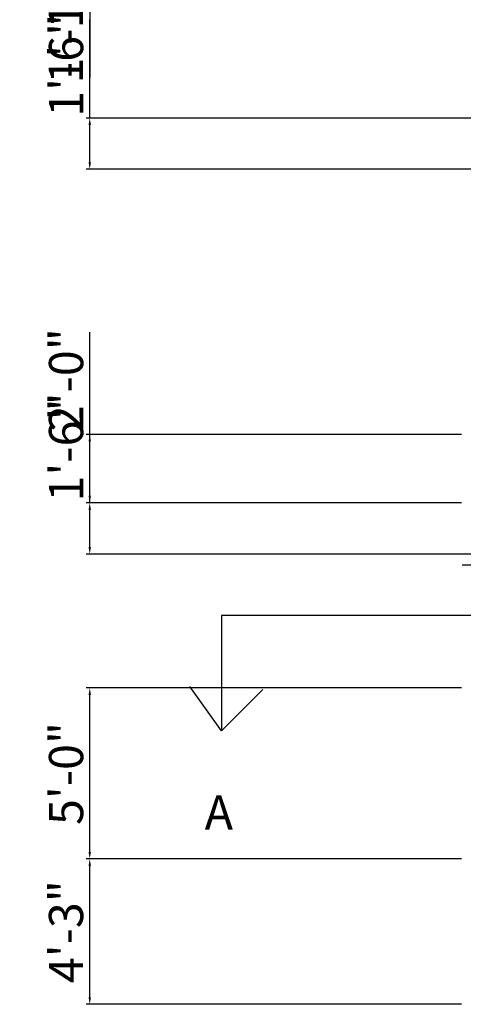
# Model space of a CAD drawing. Units: inches. Extents: x 2319 to 3765, y 2872 to 3950.
# Tile 1 of 9: x 2319 to 2474, y 2961 to 3306. Entities that reach past the tile are written whole.
import ezdxf

# ---------------------------------------------------------------- set-up
doc = ezdxf.new("R2010")
doc.units = ezdxf.units.IN
doc.layers.add('A-ANNO-DIMS', color=2, linetype='Continuous', lineweight=18)
doc.layers.add('A-ANNO-SYMB', color=3, linetype='Continuous', lineweight=25)
doc.styles.get("Standard").update_dxf_attribs({"font": 'arial.ttf'})
doc.dimstyles.new('ISO-25', dxfattribs={"dimtxt": 12, "dimasz": 2.5, "dimexe": 1.25, "dimexo": 0.625, "dimtad": 1, "dimdec": 0, "dimlunit": 3, "dimtxsty": 'Standard', "dimcen": 2.5, "dimadec": 0, "dimazin": 0, "dimtfac": 1, "dimtdec": 0, "dimtmove": 0, "dimatfit": 3, "dimfxl": 1, "dimarcsym": 0})

# ---------------------------------------------------------------- blocks, each defined once
blk = doc.blocks.new('SECTION-ARROWHEAD')
for q in [(0, 15.55), (25.55, 14.43)]:
    blk.add_line((11.08, 0), q)
blk = doc.blocks.new('*D53')
at = {"layer": 'A-ANNO-DIMS', "color": 0, "lineweight": -2, "transparency": 16777216}
for p, q in [((2604.93, 3114.7), (2473.68, 3114.7)), ((2604.93, 3111.24), (2604.93, 3115.95)), ((2629.68, 3114.7), (2607.43, 3114.7)), ((2632.18, 3111.24), (2632.18, 3115.95))]:
    blk.add_line(p, q, dxfattribs=at)
at = {"layer": 'A-ANNO-DIMS', "color": 0, "transparency": 16777216}
for points in [[(2607.43, 3115.11), (2607.43, 3114.28), (2604.93, 3114.7)], [(2629.68, 3115.11), (2629.68, 3114.28), (2632.18, 3114.7)]]:
    blk.add_solid(points, dxfattribs=at)
at = {"layer": 'Defpoints', "color": 0, "transparency": 16777216}
for p in [(2604.93, 3114.7), (2604.93, 3110.61), (2632.18, 3110.61)]:
    blk.add_point(p, dxfattribs=at)
at = {"layer": 'A-ANNO-DIMS', "color": 0, "transparency": 16777216, "insert": (2538.06, 3121.54), "char_height": 12, "attachment_point": 5}
blk.add_mtext('DOOR 2\'-3" TYP.', dxfattribs=at)
blk = doc.blocks.new('*D77')
at = {"layer": 'A-ANNO-DIMS', "color": 0, "lineweight": -2, "transparency": 16777216}
for p, q in [((2473.5, 3011.61), (2341.89, 3011.61)), ((2343.14, 2963.11), (2343.14, 3009.11)), ((2473.5, 2960.61), (2341.89, 2960.61))]:
    blk.add_line(p, q, dxfattribs=at)
at = {"layer": 'A-ANNO-DIMS', "color": 0, "transparency": 16777216}
for points in [[(2342.72, 3009.11), (2343.56, 3009.11), (2343.14, 3011.61)], [(2342.72, 2963.11), (2343.56, 2963.11), (2343.14, 2960.61)]]:
    blk.add_solid(points, dxfattribs=at)
at = {"layer": 'Defpoints', "color": 0, "transparency": 16777216}
for p in [(2343.14, 3011.61), (2474.13, 3011.61), (2474.13, 2960.61)]:
    blk.add_point(p, dxfattribs=at)
at = {"layer": 'A-ANNO-DIMS', "color": 0, "transparency": 16777216, "insert": (2336.38, 2986.11), "char_height": 12, "attachment_point": 5, "rotation": 90}
blk.add_mtext('4\'-3"', dxfattribs=at)
blk = doc.blocks.new('*D78')
at = {"layer": 'A-ANNO-DIMS', "color": 0, "lineweight": -2, "transparency": 16777216}
for p, q in [((2473.5, 3071.61), (2341.89, 3071.61)), ((2343.14, 3014.11), (2343.14, 3069.11)), ((2473.5, 3011.61), (2341.89, 3011.61))]:
    blk.add_line(p, q, dxfattribs=at)
at = {"layer": 'A-ANNO-DIMS', "color": 0, "transparency": 16777216}
for points in [[(2342.72, 3069.11), (2343.56, 3069.11), (2343.14, 3071.61)], [(2342.72, 3014.11), (2343.56, 3014.11), (2343.14, 3011.61)]]:
    blk.add_solid(points, dxfattribs=at)
at = {"layer": 'Defpoints', "color": 0, "transparency": 16777216}
for p in [(2343.14, 3071.61), (2474.13, 3071.61), (2474.13, 3011.61)]:
    blk.add_point(p, dxfattribs=at)
at = {"layer": 'A-ANNO-DIMS', "color": 0, "transparency": 16777216, "insert": (2336.39, 3041.61), "char_height": 12, "attachment_point": 5, "rotation": 90}
blk.add_mtext('5\'-0"', dxfattribs=at)
blk = doc.blocks.new('*D79')
at = {"layer": 'A-ANNO-DIMS', "color": 0, "lineweight": -2, "transparency": 16777216}
for p, q in [((2343.14, 3160.61), (2343.14, 3196.46)), ((2473.5, 3160.61), (2341.89, 3160.61)), ((2343.14, 3139.11), (2343.14, 3158.11)), ((2473.5, 3136.61), (2341.89, 3136.61))]:
    blk.add_line(p, q, dxfattribs=at)
at = {"layer": 'A-ANNO-DIMS', "color": 0, "transparency": 16777216}
for points in [[(2342.72, 3158.11), (2343.56, 3158.11), (2343.14, 3160.61)], [(2342.72, 3139.11), (2343.56, 3139.11), (2343.14, 3136.61)]]:
    blk.add_solid(points, dxfattribs=at)
at = {"layer": 'Defpoints', "color": 0, "transparency": 16777216}
for p in [(2343.14, 3160.61), (2474.13, 3160.61), (2474.13, 3136.61)]:
    blk.add_point(p, dxfattribs=at)
at = {"layer": 'A-ANNO-DIMS', "color": 0, "transparency": 16777216, "insert": (2336.39, 3179.79), "char_height": 12, "attachment_point": 5, "rotation": 90}
blk.add_mtext('2\'-0"', dxfattribs=at)
blk = doc.blocks.new('*D80')
at = {"layer": 'A-ANNO-DIMS', "color": 0, "lineweight": -2, "transparency": 16777216}
for p, q in [((2343.14, 3136.61), (2343.14, 3171.13)), ((2473.5, 3136.61), (2341.89, 3136.61)), ((2343.14, 3121.11), (2343.14, 3134.11)), ((2482.5, 3118.61), (2341.89, 3118.61))]:
    blk.add_line(p, q, dxfattribs=at)
at = {"layer": 'A-ANNO-DIMS', "color": 0, "transparency": 16777216}
for points in [[(2342.72, 3134.11), (2343.56, 3134.11), (2343.14, 3136.61)], [(2342.72, 3121.11), (2343.56, 3121.11), (2343.14, 3118.61)]]:
    blk.add_solid(points, dxfattribs=at)
at = {"layer": 'Defpoints', "color": 0, "transparency": 16777216}
for p in [(2343.14, 3136.61), (2474.13, 3136.61), (2483.13, 3118.61)]:
    blk.add_point(p, dxfattribs=at)
at = {"layer": 'A-ANNO-DIMS', "color": 0, "transparency": 16777216, "insert": (2336.39, 3155.12), "char_height": 12, "attachment_point": 5, "rotation": 90}
blk.add_mtext('1\'-6"', dxfattribs=at)
blk = doc.blocks.new('*D87')
at = {"layer": 'A-ANNO-DIMS', "color": 0, "lineweight": -2, "transparency": 16777216}
for p, q in [((2800.5, 3380.11), (2341.89, 3380.11)), ((2343.14, 3377.61), (2343.14, 3360.11)), ((2800.5, 3357.61), (2341.89, 3357.61)), ((2343.14, 3357.61), (2343.14, 3285.81))]:
    blk.add_line(p, q, dxfattribs=at)
at = {"layer": 'A-ANNO-DIMS', "color": 0, "transparency": 16777216}
for points in [[(2342.72, 3377.61), (2343.56, 3377.61), (2343.14, 3380.11)], [(2342.72, 3360.11), (2343.56, 3360.11), (2343.14, 3357.61)]]:
    blk.add_solid(points, dxfattribs=at)
at = {"layer": 'Defpoints', "color": 0, "transparency": 16777216}
for p in [(2801.13, 3380.11), (2343.14, 3357.61), (2801.13, 3357.61)]:
    blk.add_point(p, dxfattribs=at)
at = {"layer": 'A-ANNO-DIMS', "color": 0, "transparency": 16777216, "insert": (2336.31, 3320.46), "char_height": 12, "attachment_point": 5, "rotation": 90}
blk.add_mtext('1\'-10 1/2"', dxfattribs=at)
blk = doc.blocks.new('*D88')
at = {"layer": 'A-ANNO-DIMS', "color": 0, "lineweight": -2, "transparency": 16777216}
for p, q in [((2343.14, 3271.61), (2343.14, 3306.13)), ((2949.5, 3271.61), (2341.89, 3271.61)), ((2343.14, 3256.11), (2343.14, 3269.11)), ((2949.5, 3253.61), (2341.89, 3253.61))]:
    blk.add_line(p, q, dxfattribs=at)
at = {"layer": 'A-ANNO-DIMS', "color": 0, "transparency": 16777216}
for points in [[(2342.72, 3269.11), (2343.56, 3269.11), (2343.14, 3271.61)], [(2342.72, 3256.11), (2343.56, 3256.11), (2343.14, 3253.61)]]:
    blk.add_solid(points, dxfattribs=at)
at = {"layer": 'Defpoints', "color": 0, "transparency": 16777216}
for p in [(2343.14, 3271.61), (2950.13, 3271.61), (2950.13, 3253.61)]:
    blk.add_point(p, dxfattribs=at)
at = {"layer": 'A-ANNO-DIMS', "color": 0, "transparency": 16777216, "insert": (2336.39, 3290.12), "char_height": 12, "attachment_point": 5, "rotation": 90}
blk.add_mtext('1\'-6"', dxfattribs=at)

msp = doc.modelspace()

# ---------------------------------------------------------------- linework, layer by layer
at = {"layer": 'A-ANNO-SYMB'}
for p, q in [((3034.33, 3097.01), (2389.37, 3097.01)), ((2389.37, 3097.01), (2389.37, 3056.59))]:
    msp.add_line(p, q, dxfattribs=at)

# ---------------------------------------------------------------- block references
msp.add_blockref('SECTION-ARROWHEAD', (2378.29, 3056.59), dxfattribs=at)

# ---------------------------------------------------------------- texts
msp.add_text('A', height=12, dxfattribs=at).set_placement((2383.43, 3021.89))

# ---------------------------------------------------------------- dimensions: what is measured, and where the dimension line sits
at = {"layer": 'A-ANNO-DIMS'}
for base, p1, p2, picture, middle in [((2343.14, 3357.61), (2801.13, 3380.11), (2801.13, 3357.61), '*D87', (2336.31, 3320.46)), ((2343.14, 3271.61), (2950.13, 3253.61), (2950.13, 3271.61), '*D88', (2336.39, 3290.12)), ((2343.14, 3160.61), (2474.13, 3136.61), (2474.13, 3160.61), '*D79', (2336.39, 3179.79)), ((2343.14, 3136.61), (2483.13, 3118.61), (2474.13, 3136.61), '*D80', (2336.39, 3155.12)), ((2343.14, 3071.61), (2474.13, 3011.61), (2474.13, 3071.61), '*D78', (2336.39, 3041.61)), ((2343.14, 3011.61), (2474.13, 2960.61), (2474.13, 3011.61), '*D77', (2336.38, 2986.11))]:
    dim = msp.add_linear_dim(base=base, p1=p1, p2=p2, angle=90, dimstyle='ISO-25', override={"dimdec": 1, "dimlfac": 1, "dimrnd": 0, "dimzin": 1, "dimdsep": 46, "dimlunit": 4, "dimfrac": 2}, dxfattribs=at)
    dim.commit()
    dim.dimension.update_dxf_attribs({"geometry": picture, "text_midpoint": middle})
dim = msp.add_linear_dim(base=(2604.9322, 3114.6979), p1=(2632.1792, 3110.6109), p2=(2604.9322, 3110.6109), angle=180, text='DOOR <> TYP.', dimstyle='ISO-25', override={"dimdec": 1, "dimlfac": 1, "dimrnd": 0, "dimzin": 1, "dimdsep": 46, "dimlunit": 4, "dimfrac": 2}, dxfattribs=at)
dim.commit()
dim.dimension.update_dxf_attribs({"geometry": '*D53', "text_midpoint": (2538.0583, 3121.5357)})

doc.saveas('drawing.dxf')
